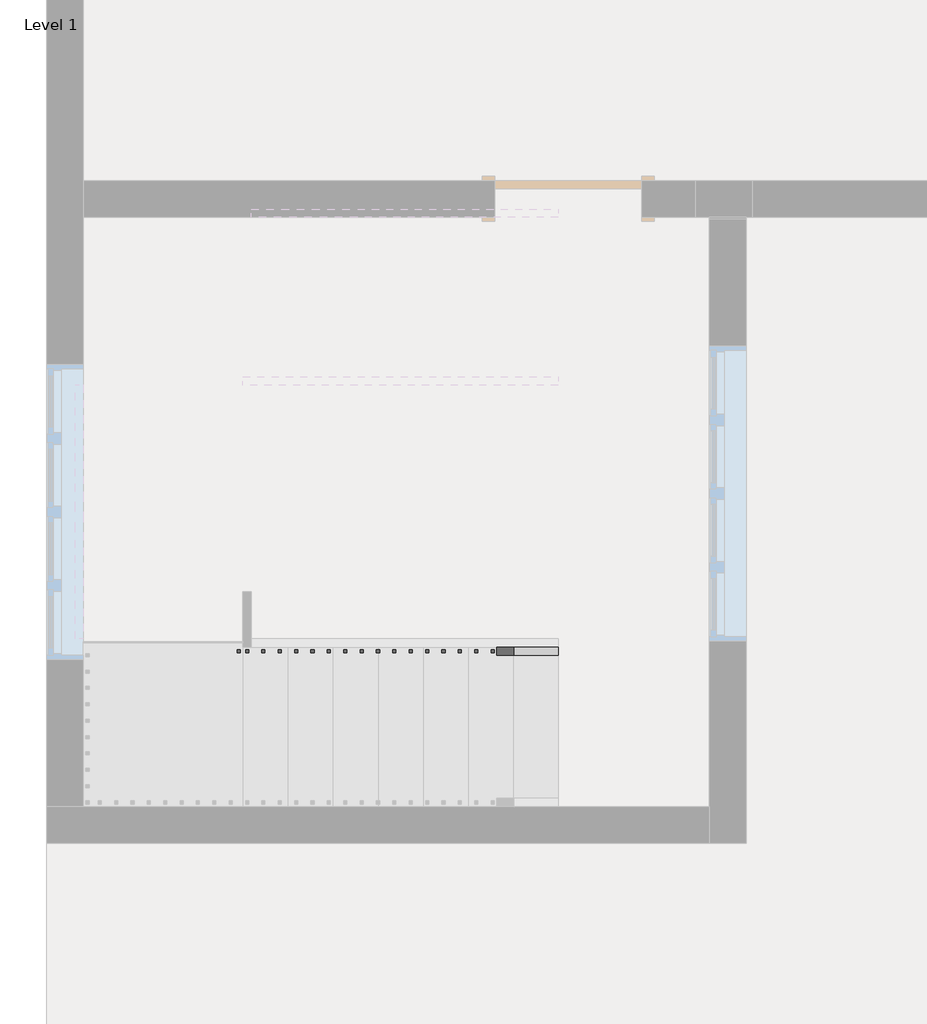
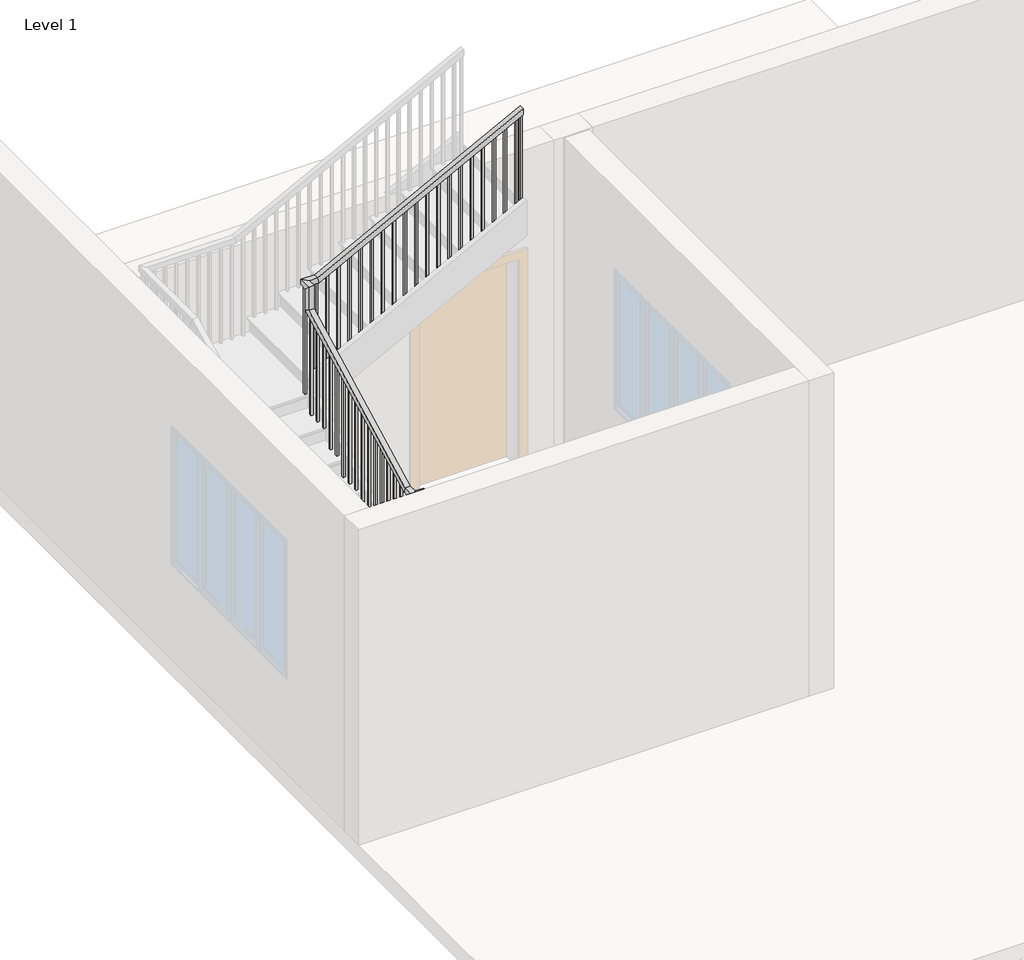
# One storey, part 6 of 8: 1 railing.
"""IFC4 building model written with IfcOpenShell, lengths in millimetres."""

from ifc_helpers import new_model, si_unit, frame, origin, place, context, project, spatial, polyline, outline, extrude, faceted_brep, element, save

model = new_model("IFC4")

# Units and contexts
model_context = context("Model", 3, world=origin())
ifc_project = project(units=[si_unit("LENGTHUNIT", "METRE", prefix="MILLI")], contexts=[model_context])

# Site, building, storey
site = spatial("IfcSite", under=ifc_project)
building = spatial("IfcBuilding", under=site)
storey = spatial("IfcBuildingStorey", under=building, Name="Level 1", Elevation=0.0)

# Railing
placement = place(None, origin())
element("IfcRailing", 1, ObjectType="Handrail - Rectangular", at=placement, inside=storey, context=model_context, shape_type="SolidModel", body=[
    faceted_brep([(14750.242447, -178.6399287, 1059.5428571), (14750.242447, -178.6399287, 1002.2973199), (14750.242447, -127.8399287, 1002.2973199), (14750.242447, -127.8399287, 1059.5428571), (12870.642447, -178.6399287, 2035.9584416), (12819.842447, -178.6399287, 2005.1025147), (12819.842447, -127.8399287, 2005.1025147), (12870.642447, -127.8399287, 2035.9584416), (12743.642447, -39.2322695, 2209.4701299), (12743.642447, -51.6399287, 2260.2701299), (12743.642447, 1472.3600713, 3051.9584416), (12743.642447, 1523.1600713, 3021.1025147), (12794.442447, -39.2322695, 2209.4701299), (12794.442447, 1523.1600713, 3021.1025147), (12794.442447, -51.6399287, 2260.2701299), (12794.442447, 1472.3600713, 3051.9584416), (14750.242447, 1599.3600713, 4252.6857143), (14750.242447, 1548.5600713, 4252.6857143), (14750.242447, 1548.5600713, 4195.440177), (14750.242447, 1599.3600713, 4195.440177), (12883.0501063, 1599.3600713, 3225.4701299), (12870.642447, 1599.3600713, 3276.2701299), (12883.0501063, 1548.5600713, 3225.4701299), (12870.642447, 1548.5600713, 3276.2701299), (12870.642447, -178.6399287, 2260.2701299), (12819.842447, -178.6399287, 2209.4701299), (12819.842447, -127.8399287, 2209.4701299), (12870.642447, -127.8399287, 2260.2701299), (12743.642447, -178.6399287, 2260.2701299), (12743.642447, -178.6399287, 2209.4701299), (12794.442447, -127.8399287, 2209.4701299), (12794.442447, -127.8399287, 2260.2701299), (12743.642447, 1472.3600713, 3276.2701299), (12743.642447, 1523.1600713, 3225.4701299), (12794.442447, 1523.1600713, 3225.4701299), (12794.442447, 1472.3600713, 3276.2701299), (12743.642447, 1599.3600713, 3276.2701299), (12743.642447, 1599.3600713, 3225.4701299), (12794.442447, 1548.5600713, 3225.4701299), (12794.442447, 1548.5600713, 3276.2701299)], [[[0, 1, 2, 3]], [[1, 0, 4, 5]], [[2, 1, 5, 6]], [[3, 2, 6, 7]], [[0, 3, 7, 4]], [[8, 9, 10, 11]], [[12, 8, 11, 13]], [[14, 12, 13, 15]], [[9, 14, 15, 10]], [[16, 17, 18, 19]], [[20, 21, 16, 19]], [[22, 20, 19, 18]], [[23, 22, 18, 17]], [[21, 23, 17, 16]], [[5, 4, 24, 25]], [[6, 5, 25, 26]], [[7, 6, 26, 27]], [[4, 7, 27, 24]], [[25, 24, 28, 29]], [[26, 25, 29, 30]], [[27, 26, 30, 31]], [[24, 27, 31, 28]], [[29, 28, 9, 8]], [[30, 29, 8, 12]], [[31, 30, 12, 14]], [[28, 31, 14, 9]], [[11, 10, 32, 33]], [[13, 11, 33, 34]], [[15, 13, 34, 35]], [[10, 15, 35, 32]], [[33, 32, 36, 37]], [[34, 33, 37, 38]], [[35, 34, 38, 39]], [[32, 35, 39, 36]], [[37, 36, 21, 20]], [[38, 37, 20, 22]], [[39, 38, 22, 23]], [[36, 39, 23, 21]]]),
    extrude(outline(polyline([(4173.9986186, 14708.967447), (4164.1025147, 14689.917447), (3193.1428571, 14689.917447), (3193.1428571, 14708.967447), (4173.9986186, 14708.967447)])), frame((0.0, 1564.4350713, 0.0), z_axis=(0.0, 1.0, 0.0), x_axis=(0.0, 0.0, 1.0)), (0.0, 0.0, 1.0), 19.05),
    extrude(outline(polyline([(4121.2193978, 14607.367447), (4111.3232939, 14588.317447), (3193.1428571, 14588.317447), (3193.1428571, 14607.367447), (4121.2193978, 14607.367447)])), frame((0.0, 1564.4350713, 0.0), z_axis=(0.0, 1.0, 0.0), x_axis=(0.0, 0.0, 1.0)), (0.0, 0.0, 1.0), 19.05),
    extrude(outline(polyline([(4068.440177, 14505.767447), (4058.5440731, 14486.717447), (3193.1428571, 14486.717447), (3193.1428571, 14505.767447), (4068.440177, 14505.767447)])), frame((0.0, 1564.4350713, 0.0), z_axis=(0.0, 1.0, 0.0), x_axis=(0.0, 0.0, 1.0)), (0.0, 0.0, 1.0), 19.05),
    extrude(outline(polyline([(4015.6609562, 14404.167447), (4005.7648523, 14385.117447), (3048.0, 14385.117447), (3048.0, 14404.167447), (4015.6609562, 14404.167447)])), frame((0.0, 1564.4350713, 0.0), z_axis=(0.0, 1.0, 0.0), x_axis=(0.0, 0.0, 1.0)), (0.0, 0.0, 1.0), 19.05),
    extrude(outline(polyline([(3962.8817355, 14302.567447), (3952.9856316, 14283.517447), (3048.0, 14283.517447), (3048.0, 14302.567447), (3962.8817355, 14302.567447)])), frame((0.0, 1564.4350713, 0.0), z_axis=(0.0, 1.0, 0.0), x_axis=(0.0, 0.0, 1.0)), (0.0, 0.0, 1.0), 19.05),
    extrude(outline(polyline([(3910.1025147, 14200.967447), (3900.2064108, 14181.917447), (3048.0, 14181.917447), (3048.0, 14200.967447), (3910.1025147, 14200.967447)])), frame((0.0, 1564.4350713, 0.0), z_axis=(0.0, 1.0, 0.0), x_axis=(0.0, 0.0, 1.0)), (0.0, 0.0, 1.0), 19.05),
    extrude(outline(polyline([(3857.3232939, 14099.367447), (3847.42719, 14080.317447), (2902.8571429, 14080.317447), (2902.8571429, 14099.367447), (3857.3232939, 14099.367447)])), frame((0.0, 1564.4350713, 0.0), z_axis=(0.0, 1.0, 0.0), x_axis=(0.0, 0.0, 1.0)), (0.0, 0.0, 1.0), 19.05),
    extrude(outline(polyline([(3804.5440731, 13997.767447), (3794.6479692, 13978.717447), (2902.8571429, 13978.717447), (2902.8571429, 13997.767447), (3804.5440731, 13997.767447)])), frame((0.0, 1564.4350713, 0.0), z_axis=(0.0, 1.0, 0.0), x_axis=(0.0, 0.0, 1.0)), (0.0, 0.0, 1.0), 19.05),
    extrude(outline(polyline([(3751.7648523, 13896.167447), (3741.8687485, 13877.117447), (2757.7142857, 13877.117447), (2757.7142857, 13896.167447), (3751.7648523, 13896.167447)])), frame((0.0, 1564.4350713, 0.0), z_axis=(0.0, 1.0, 0.0), x_axis=(0.0, 0.0, 1.0)), (0.0, 0.0, 1.0), 19.05),
    extrude(outline(polyline([(3698.9856316, 13794.567447), (3689.0895277, 13775.517447), (2757.7142857, 13775.517447), (2757.7142857, 13794.567447), (3698.9856316, 13794.567447)])), frame((0.0, 1564.4350713, 0.0), z_axis=(0.0, 1.0, 0.0), x_axis=(0.0, 0.0, 1.0)), (0.0, 0.0, 1.0), 19.05),
    extrude(outline(polyline([(3646.2064108, 13692.967447), (3636.3103069, 13673.917447), (2757.7142857, 13673.917447), (2757.7142857, 13692.967447), (3646.2064108, 13692.967447)])), frame((0.0, 1564.4350713, 0.0), z_axis=(0.0, 1.0, 0.0), x_axis=(0.0, 0.0, 1.0)), (0.0, 0.0, 1.0), 19.05),
    extrude(outline(polyline([(3593.42719, 13591.367447), (3583.5310861, 13572.317447), (2612.5714286, 13572.317447), (2612.5714286, 13591.367447), (3593.42719, 13591.367447)])), frame((0.0, 1564.4350713, 0.0), z_axis=(0.0, 1.0, 0.0), x_axis=(0.0, 0.0, 1.0)), (0.0, 0.0, 1.0), 19.05),
    extrude(outline(polyline([(3540.6479692, 13489.767447), (3530.7518653, 13470.717447), (2612.5714286, 13470.717447), (2612.5714286, 13489.767447), (3540.6479692, 13489.767447)])), frame((0.0, 1564.4350713, 0.0), z_axis=(0.0, 1.0, 0.0), x_axis=(0.0, 0.0, 1.0)), (0.0, 0.0, 1.0), 19.05),
    extrude(outline(polyline([(3487.8687485, 13388.167447), (3477.9726446, 13369.117447), (2612.5714286, 13369.117447), (2612.5714286, 13388.167447), (3487.8687485, 13388.167447)])), frame((0.0, 1564.4350713, 0.0), z_axis=(0.0, 1.0, 0.0), x_axis=(0.0, 0.0, 1.0)), (0.0, 0.0, 1.0), 19.05),
    extrude(outline(polyline([(3435.0895277, 13286.567447), (3425.1934238, 13267.517447), (2467.4285714, 13267.517447), (2467.4285714, 13286.567447), (3435.0895277, 13286.567447)])), frame((0.0, 1564.4350713, 0.0), z_axis=(0.0, 1.0, 0.0), x_axis=(0.0, 0.0, 1.0)), (0.0, 0.0, 1.0), 19.05),
    extrude(outline(polyline([(3382.3103069, 13184.967447), (3372.414203, 13165.917447), (2467.4285714, 13165.917447), (2467.4285714, 13184.967447), (3382.3103069, 13184.967447)])), frame((0.0, 1564.4350713, 0.0), z_axis=(0.0, 1.0, 0.0), x_axis=(0.0, 0.0, 1.0)), (0.0, 0.0, 1.0), 19.05),
    extrude(outline(polyline([(3329.5310861, 13083.367447), (3319.6349822, 13064.317447), (2467.4285714, 13064.317447), (2467.4285714, 13083.367447), (3329.5310861, 13083.367447)])), frame((0.0, 1564.4350713, 0.0), z_axis=(0.0, 1.0, 0.0), x_axis=(0.0, 0.0, 1.0)), (0.0, 0.0, 1.0), 19.05),
    extrude(outline(polyline([(3276.7518653, 12981.767447), (3266.8557614, 12962.717447), (2322.2857143, 12962.717447), (2322.2857143, 12981.767447), (3276.7518653, 12981.767447)])), frame((0.0, 1564.4350713, 0.0), z_axis=(0.0, 1.0, 0.0), x_axis=(0.0, 0.0, 1.0)), (0.0, 0.0, 1.0), 19.05),
    extrude(outline(polyline([(3223.9726446, 12880.167447), (3214.0765407, 12861.117447), (2322.2857143, 12861.117447), (2322.2857143, 12880.167447), (3223.9726446, 12880.167447)])), frame((0.0, 1564.4350713, 0.0), z_axis=(0.0, 1.0, 0.0), x_axis=(0.0, 0.0, 1.0)), (0.0, 0.0, 1.0), 19.05),
    extrude(outline(polyline([(1462.8350713, 2989.7648523), (1481.8850713, 2999.6609562), (1481.8850713, 2032.0), (1462.8350713, 2032.0), (1462.8350713, 2989.7648523)])), frame((12759.517447, 0.0, 0.0), z_axis=(1.0, 0.0, 0.0), x_axis=(0.0, 1.0, 0.0)), (0.0, 0.0, 1.0), 19.05),
    extrude(outline(polyline([(1361.2350713, 2936.9856316), (1380.2850713, 2946.8817355), (1380.2850713, 2032.0), (1361.2350713, 2032.0), (1361.2350713, 2936.9856316)])), frame((12759.517447, 0.0, 0.0), z_axis=(1.0, 0.0, 0.0), x_axis=(0.0, 1.0, 0.0)), (0.0, 0.0, 1.0), 19.05),
    extrude(outline(polyline([(1259.6350713, 2884.2064108), (1278.6850713, 2894.1025147), (1278.6850713, 2032.0), (1259.6350713, 2032.0), (1259.6350713, 2884.2064108)])), frame((12759.517447, 0.0, 0.0), z_axis=(1.0, 0.0, 0.0), x_axis=(0.0, 1.0, 0.0)), (0.0, 0.0, 1.0), 19.05),
    extrude(outline(polyline([(1158.0350713, 2831.42719), (1177.0850713, 2841.3232939), (1177.0850713, 1886.8571429), (1158.0350713, 1886.8571429), (1158.0350713, 2831.42719)])), frame((12759.517447, 0.0, 0.0), z_axis=(1.0, 0.0, 0.0), x_axis=(0.0, 1.0, 0.0)), (0.0, 0.0, 1.0), 19.05),
    extrude(outline(polyline([(1056.4350713, 2778.6479692), (1075.4850713, 2788.5440731), (1075.4850713, 1886.8571429), (1056.4350713, 1886.8571429), (1056.4350713, 2778.6479692)])), frame((12759.517447, 0.0, 0.0), z_axis=(1.0, 0.0, 0.0), x_axis=(0.0, 1.0, 0.0)), (0.0, 0.0, 1.0), 19.05),
    extrude(outline(polyline([(954.8350713, 2725.8687485), (973.8850713, 2735.7648523), (973.8850713, 1741.7142857), (954.8350713, 1741.7142857), (954.8350713, 2725.8687485)])), frame((12759.517447, 0.0, 0.0), z_axis=(1.0, 0.0, 0.0), x_axis=(0.0, 1.0, 0.0)), (0.0, 0.0, 1.0), 19.05),
    extrude(outline(polyline([(853.2350713, 2673.0895277), (872.2850713, 2682.9856316), (872.2850713, 1741.7142857), (853.2350713, 1741.7142857), (853.2350713, 2673.0895277)])), frame((12759.517447, 0.0, 0.0), z_axis=(1.0, 0.0, 0.0), x_axis=(0.0, 1.0, 0.0)), (0.0, 0.0, 1.0), 19.05),
    extrude(outline(polyline([(751.6350713, 2620.3103069), (770.6850713, 2630.2064108), (770.6850713, 1741.7142857), (751.6350713, 1741.7142857), (751.6350713, 2620.3103069)])), frame((12759.517447, 0.0, 0.0), z_axis=(1.0, 0.0, 0.0), x_axis=(0.0, 1.0, 0.0)), (0.0, 0.0, 1.0), 19.05),
    extrude(outline(polyline([(650.0350713, 2567.5310861), (669.0850713, 2577.42719), (669.0850713, 1596.5714286), (650.0350713, 1596.5714286), (650.0350713, 2567.5310861)])), frame((12759.517447, 0.0, 0.0), z_axis=(1.0, 0.0, 0.0), x_axis=(0.0, 1.0, 0.0)), (0.0, 0.0, 1.0), 19.05),
    extrude(outline(polyline([(548.4350713, 2514.7518653), (567.4850713, 2524.6479692), (567.4850713, 1596.5714286), (548.4350713, 1596.5714286), (548.4350713, 2514.7518653)])), frame((12759.517447, 0.0, 0.0), z_axis=(1.0, 0.0, 0.0), x_axis=(0.0, 1.0, 0.0)), (0.0, 0.0, 1.0), 19.05),
    extrude(outline(polyline([(446.8350713, 2461.9726446), (465.8850713, 2471.8687485), (465.8850713, 1596.5714286), (446.8350713, 1596.5714286), (446.8350713, 2461.9726446)])), frame((12759.517447, 0.0, 0.0), z_axis=(1.0, 0.0, 0.0), x_axis=(0.0, 1.0, 0.0)), (0.0, 0.0, 1.0), 19.05),
    extrude(outline(polyline([(345.2350713, 2409.1934238), (364.2850713, 2419.0895277), (364.2850713, 1451.4285714), (345.2350713, 1451.4285714), (345.2350713, 2409.1934238)])), frame((12759.517447, 0.0, 0.0), z_axis=(1.0, 0.0, 0.0), x_axis=(0.0, 1.0, 0.0)), (0.0, 0.0, 1.0), 19.05),
    extrude(outline(polyline([(243.6350713, 2356.414203), (262.6850713, 2366.3103069), (262.6850713, 1451.4285714), (243.6350713, 1451.4285714), (243.6350713, 2356.414203)])), frame((12759.517447, 0.0, 0.0), z_axis=(1.0, 0.0, 0.0), x_axis=(0.0, 1.0, 0.0)), (0.0, 0.0, 1.0), 19.05),
    extrude(outline(polyline([(142.0350713, 2303.6349822), (161.0850713, 2313.5310861), (161.0850713, 1451.4285714), (142.0350713, 1451.4285714), (142.0350713, 2303.6349822)])), frame((12759.517447, 0.0, 0.0), z_axis=(1.0, 0.0, 0.0), x_axis=(0.0, 1.0, 0.0)), (0.0, 0.0, 1.0), 19.05),
    extrude(outline(polyline([(40.4350713, 2250.8557614), (59.4850713, 2260.7518653), (59.4850713, 1306.2857143), (40.4350713, 1306.2857143), (40.4350713, 2250.8557614)])), frame((12759.517447, 0.0, 0.0), z_axis=(1.0, 0.0, 0.0), x_axis=(0.0, 1.0, 0.0)), (0.0, 0.0, 1.0), 19.05),
    extrude(outline(polyline([(-61.1649287, 2198.0765407), (-42.1149287, 2207.9726446), (-42.1149287, 1306.2857143), (-61.1649287, 1306.2857143), (-61.1649287, 2198.0765407)])), frame((12759.517447, 0.0, 0.0), z_axis=(1.0, 0.0, 0.0), x_axis=(0.0, 1.0, 0.0)), (0.0, 0.0, 1.0), 19.05),
    extrude(outline(polyline([(12829.367447, -143.7149287), (12829.367447, -162.7649287), (12810.317447, -162.7649287), (12810.317447, -143.7149287), (12829.367447, -143.7149287)])), frame((0.0, 0.0, 1016.0), z_axis=(0.0, 0.0, 1.0), x_axis=(1.0, 0.0, 0.0)), (0.0, 0.0, 1.0), 1193.4701299),
    extrude(outline(polyline([(1947.375242, 12930.967447), (1957.2713459, 12911.917447), (1016.0, 12911.917447), (1016.0, 12930.967447), (1947.375242, 12930.967447)])), frame((0.0, -162.7649287, 0.0), z_axis=(0.0, 1.0, 0.0), x_axis=(0.0, 0.0, 1.0)), (0.0, 0.0, 1.0), 19.05),
    extrude(outline(polyline([(1894.5960212, 13032.567447), (1904.4921251, 13013.517447), (1016.0, 13013.517447), (1016.0, 13032.567447), (1894.5960212, 13032.567447)])), frame((0.0, -162.7649287, 0.0), z_axis=(0.0, 1.0, 0.0), x_axis=(0.0, 0.0, 1.0)), (0.0, 0.0, 1.0), 19.05),
    extrude(outline(polyline([(1841.8168004, 13134.167447), (1851.7129043, 13115.117447), (870.8571429, 13115.117447), (870.8571429, 13134.167447), (1841.8168004, 13134.167447)])), frame((0.0, -162.7649287, 0.0), z_axis=(0.0, 1.0, 0.0), x_axis=(0.0, 0.0, 1.0)), (0.0, 0.0, 1.0), 19.05),
    extrude(outline(polyline([(1789.0375796, 13235.767447), (1798.9336835, 13216.717447), (870.8571429, 13216.717447), (870.8571429, 13235.767447), (1789.0375796, 13235.767447)])), frame((0.0, -162.7649287, 0.0), z_axis=(0.0, 1.0, 0.0), x_axis=(0.0, 0.0, 1.0)), (0.0, 0.0, 1.0), 19.05),
    extrude(outline(polyline([(1736.2583588, 13337.367447), (1746.1544627, 13318.317447), (870.8571429, 13318.317447), (870.8571429, 13337.367447), (1736.2583588, 13337.367447)])), frame((0.0, -162.7649287, 0.0), z_axis=(0.0, 1.0, 0.0), x_axis=(0.0, 0.0, 1.0)), (0.0, 0.0, 1.0), 19.05),
    extrude(outline(polyline([(1683.4791381, 13438.967447), (1693.375242, 13419.917447), (725.7142857, 13419.917447), (725.7142857, 13438.967447), (1683.4791381, 13438.967447)])), frame((0.0, -162.7649287, 0.0), z_axis=(0.0, 1.0, 0.0), x_axis=(0.0, 0.0, 1.0)), (0.0, 0.0, 1.0), 19.05),
    extrude(outline(polyline([(1630.6999173, 13540.567447), (1640.5960212, 13521.517447), (725.7142857, 13521.517447), (725.7142857, 13540.567447), (1630.6999173, 13540.567447)])), frame((0.0, -162.7649287, 0.0), z_axis=(0.0, 1.0, 0.0), x_axis=(0.0, 0.0, 1.0)), (0.0, 0.0, 1.0), 19.05),
    extrude(outline(polyline([(1577.9206965, 13642.167447), (1587.8168004, 13623.117447), (725.7142857, 13623.117447), (725.7142857, 13642.167447), (1577.9206965, 13642.167447)])), frame((0.0, -162.7649287, 0.0), z_axis=(0.0, 1.0, 0.0), x_axis=(0.0, 0.0, 1.0)), (0.0, 0.0, 1.0), 19.05),
    extrude(outline(polyline([(1525.1414757, 13743.767447), (1535.0375796, 13724.717447), (580.5714286, 13724.717447), (580.5714286, 13743.767447), (1525.1414757, 13743.767447)])), frame((0.0, -162.7649287, 0.0), z_axis=(0.0, 1.0, 0.0), x_axis=(0.0, 0.0, 1.0)), (0.0, 0.0, 1.0), 19.05),
    extrude(outline(polyline([(1472.3622549, 13845.367447), (1482.2583588, 13826.317447), (580.5714286, 13826.317447), (580.5714286, 13845.367447), (1472.3622549, 13845.367447)])), frame((0.0, -162.7649287, 0.0), z_axis=(0.0, 1.0, 0.0), x_axis=(0.0, 0.0, 1.0)), (0.0, 0.0, 1.0), 19.05),
    extrude(outline(polyline([(1419.5830342, 13946.967447), (1429.4791381, 13927.917447), (435.4285714, 13927.917447), (435.4285714, 13946.967447), (1419.5830342, 13946.967447)])), frame((0.0, -162.7649287, 0.0), z_axis=(0.0, 1.0, 0.0), x_axis=(0.0, 0.0, 1.0)), (0.0, 0.0, 1.0), 19.05),
    extrude(outline(polyline([(1366.8038134, 14048.567447), (1376.6999173, 14029.517447), (435.4285714, 14029.517447), (435.4285714, 14048.567447), (1366.8038134, 14048.567447)])), frame((0.0, -162.7649287, 0.0), z_axis=(0.0, 1.0, 0.0), x_axis=(0.0, 0.0, 1.0)), (0.0, 0.0, 1.0), 19.05),
    extrude(outline(polyline([(1314.0245926, 14150.167447), (1323.9206965, 14131.117447), (435.4285714, 14131.117447), (435.4285714, 14150.167447), (1314.0245926, 14150.167447)])), frame((0.0, -162.7649287, 0.0), z_axis=(0.0, 1.0, 0.0), x_axis=(0.0, 0.0, 1.0)), (0.0, 0.0, 1.0), 19.05),
    extrude(outline(polyline([(1261.2453718, 14251.767447), (1271.1414757, 14232.717447), (290.2857143, 14232.717447), (290.2857143, 14251.767447), (1261.2453718, 14251.767447)])), frame((0.0, -162.7649287, 0.0), z_axis=(0.0, 1.0, 0.0), x_axis=(0.0, 0.0, 1.0)), (0.0, 0.0, 1.0), 19.05),
    extrude(outline(polyline([(1208.466151, 14353.367447), (1218.3622549, 14334.317447), (290.2857143, 14334.317447), (290.2857143, 14353.367447), (1208.466151, 14353.367447)])), frame((0.0, -162.7649287, 0.0), z_axis=(0.0, 1.0, 0.0), x_axis=(0.0, 0.0, 1.0)), (0.0, 0.0, 1.0), 19.05),
    extrude(outline(polyline([(1155.6869303, 14454.967447), (1165.5830342, 14435.917447), (290.2857143, 14435.917447), (290.2857143, 14454.967447), (1155.6869303, 14454.967447)])), frame((0.0, -162.7649287, 0.0), z_axis=(0.0, 1.0, 0.0), x_axis=(0.0, 0.0, 1.0)), (0.0, 0.0, 1.0), 19.05),
    extrude(outline(polyline([(1102.9077095, 14556.567447), (1112.8038134, 14537.517447), (145.1428571, 14537.517447), (145.1428571, 14556.567447), (1102.9077095, 14556.567447)])), frame((0.0, -162.7649287, 0.0), z_axis=(0.0, 1.0, 0.0), x_axis=(0.0, 0.0, 1.0)), (0.0, 0.0, 1.0), 19.05),
    extrude(outline(polyline([(1050.1284887, 14658.167447), (1060.0245926, 14639.117447), (145.1428571, 14639.117447), (145.1428571, 14658.167447), (1050.1284887, 14658.167447)])), frame((0.0, -162.7649287, 0.0), z_axis=(0.0, 1.0, 0.0), x_axis=(0.0, 0.0, 1.0)), (0.0, 0.0, 1.0), 19.05),
    extrude(outline(polyline([(12778.567447, 1564.4350713), (12759.517447, 1564.4350713), (12759.517447, 1583.4850713), (12778.567447, 1583.4850713), (12778.567447, 1564.4350713)])), frame((0.0, 0.0, 2177.1428571), z_axis=(0.0, 0.0, 1.0), x_axis=(1.0, 0.0, 0.0)), (0.0, 0.0, 1.0), 1048.3272727),
    extrude(outline(polyline([(12778.567447, -143.7149287), (12778.567447, -162.7649287), (12759.517447, -162.7649287), (12759.517447, -143.7149287), (12778.567447, -143.7149287)])), frame((0.0, 0.0, 1161.1428571), z_axis=(0.0, 0.0, 1.0), x_axis=(1.0, 0.0, 0.0)), (0.0, 0.0, 1.0), 1048.3272727),
    extrude(outline(polyline([(4195.440177, 14750.242447), (4185.5440731, 14731.192447), (3193.1428571, 14731.192447), (3193.1428571, 14750.242447), (4195.440177, 14750.242447)])), frame((0.0, 1564.4350713, 0.0), z_axis=(0.0, 1.0, 0.0), x_axis=(0.0, 0.0, 1.0)), (0.0, 0.0, 1.0), 19.05),
    extrude(outline(polyline([(1002.2973199, 14750.242447), (1012.1934238, 14731.192447), (145.1428571, 14731.192447), (145.1428571, 14750.242447), (1002.2973199, 14750.242447)])), frame((0.0, -162.7649287, 0.0), z_axis=(0.0, 1.0, 0.0), x_axis=(0.0, 0.0, 1.0)), (0.0, 0.0, 1.0), 19.05),
])

save(model, "model.ifc")

# Revit data of these elements
# Type "Handrail - Rectangular"
#   Assembly Code = "C2010400"
#   built-in parameter 1008612 = 0.0416667 (stored number, unit not read)
#   built-in parameter 1008611 = 0.0416667 (stored number, unit not read)
#   built-in parameter 1008609 = 0.333333 (stored number, unit not read)
#   built-in parameter 1008604 = 0.166667 (stored number, unit not read)
#   built-in parameter 1008603 = 0.166667 (stored number, unit not read)
#   Railing Height = 3' - 0"
#   built-in parameter 1008630 = 2
#   built-in parameter 1008610 = 2
#   built-in parameter 1008618 = Baluster - Square : 3/4"
# Element 1 (IfcRailing, "Handrail - Rectangular")
#   Phase Created = New Construction
